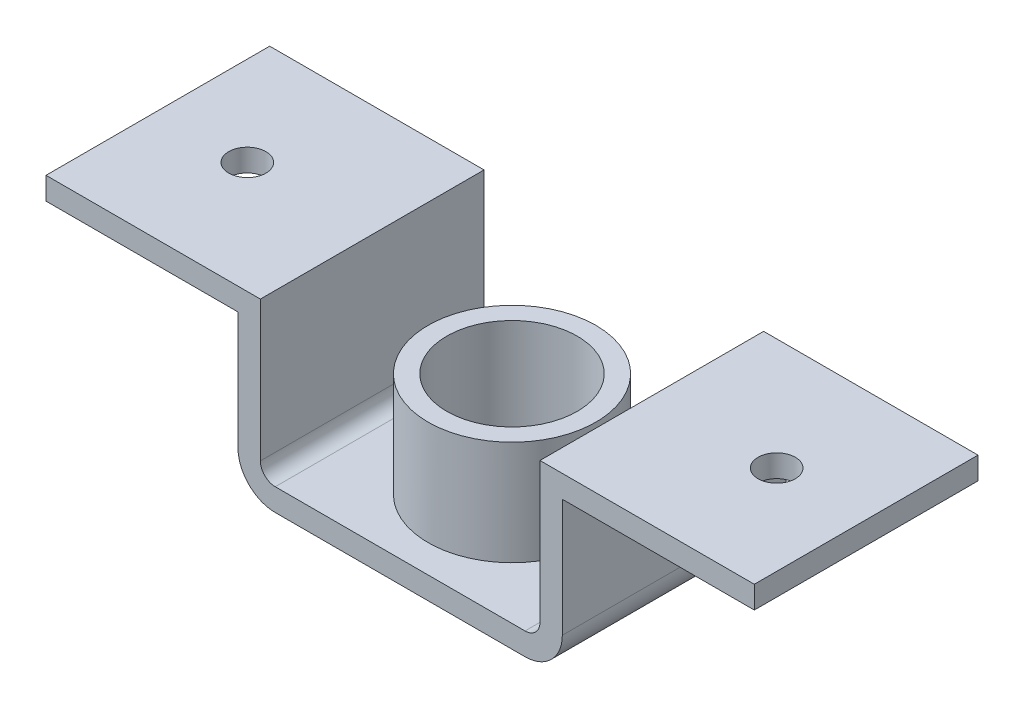
SolidWorks part; units mm, degrees
material "Plain Carbon Steel"
ref_plane "Front Plane" through (0, 0, 0) normal (0, 0, 1) x (1, 0, 0)
ref_plane "Top Plane" through (0, 0, 0) normal (0, 1, 0) x (1, 0, 0)
ref_plane "Right Plane" through (0, 0, 0) normal (1, 0, 0) x (0, 0, -1)
sketch "Bracket Profile Sketch" plane through (0, 0, 0) normal (0, 0, 1) x (1, 0, 0)
  line L0 (-475, 208) -> (-187.5, 208)
  line L1 (-187.5, 208) -> (-187.5, 0)
  line L2 (-187.5, 0) -> (187.5, 0)
  line L3 (187.5, 0) -> (187.5, 208)
  line L4 (187.5, 208) -> (475, 208)
  line L5 (0, 0) -> (0, 303.587) construction
  line L6 (-475, 178) -> (-217.5, 178)
  line L7 (-217.5, 178) -> (-217.5, -30)
  line L8 (-217.5, -30) -> (217.5, -30)
  line L9 (217.5, -30) -> (217.5, 178)
  line L10 (217.5, 178) -> (475, 178)
  line L11 (-475, 178) -> (-475, 208)
  line L12 (475, 178) -> (475, 208)
  dimension "D1" = 950
  dimension "D2" = 375
  dimension "D4" = 238
  dimension "D3" = 30
extrude "Z Bracket Body" add sketch "Bracket Profile Sketch" along normal mid plane 300
sketch "Tube Boss Sketch" plane through (0, 0, 0) normal (0, 1, 0) x (1, 0, 0)
  circle A0 centre (0, 0) radius 112.5
  circle A1 centre (0, 0) radius 87.5
  dimension "D1" = 225
  dimension "D2" = 175
extrude "Tube Boss Ø225xØ175" add sketch "Tube Boss Sketch" along normal blind 140
sketch "Centre Hole Sketch" plane through (0, 0, 0) normal (0, 1, 0) x (1, 0, 0)
  circle A0 centre (0, 0) radius 37.5
  dimension "D1" = 75
extrude "Centre Hole Ø75" cut sketch "Centre Hole Sketch" against normal blind 140
sketch "Flange Holes Sketch" plane through (0, 208, 0) normal (0, 1, 0) x (1, 0, 0)
  line L0 (-475, -150) -> (-475, 150) construction
  line L1 (-187.5, -150) -> (-475, -150) construction
  line L2 (0, -130.9) -> (0, 130.9) construction
  circle A0 centre (-355, 0) radius 25
  circle A1 centre (355, 0) radius 25
  dimension "D1" = 50
  dimension "D2" = 120
  dimension "D3" = 150
extrude "Flange Mounting Holes" cut sketch "Flange Holes Sketch" against normal blind 140
fillet "Bend Fillet R20" radius 20 2 edges at (187.5, 0, 0) (-187.5, 0, 0)
fillet "Bend Fillet R50" radius 50 2 edges at (217.5, -30, 0) (-217.5, -30, 0)
